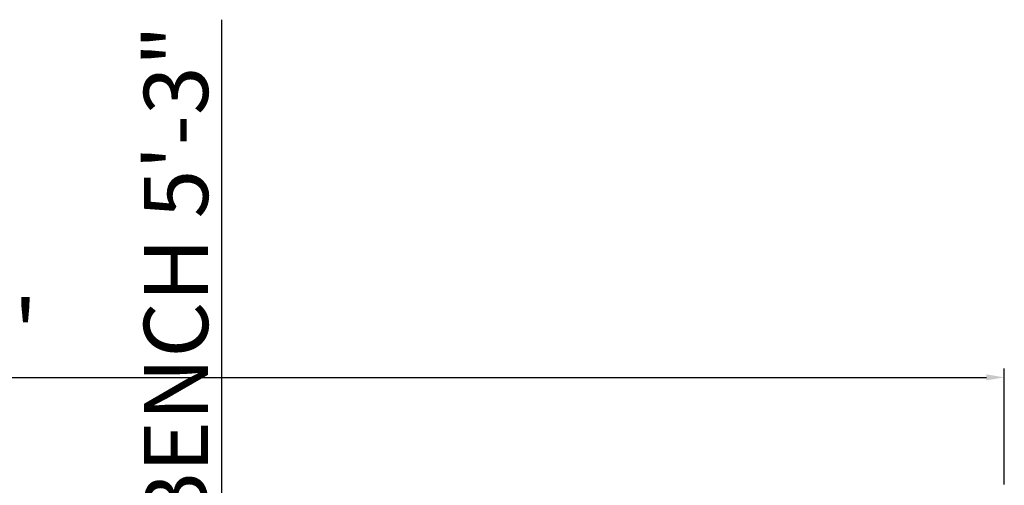
# Model space of a CAD drawing. Units: inches. Extents: x 3148 to 3962, y 1142 to 1671.
# Tile 6 of 9: x 3344 to 3482, y 1555 to 1621. Entities that reach past the tile are written whole.
import ezdxf

# ---------------------------------------------------------------- set-up
doc = ezdxf.new("R2010")
doc.units = ezdxf.units.IN
doc.layers.add('A-ANNO-DIMS', color=2, linetype='Continuous', lineweight=18)
doc.styles.get("Standard").update_dxf_attribs({"font": 'arial.ttf'})
doc.dimstyles.new('ISO-25', dxfattribs={"dimtxt": 9, "dimasz": 2.5, "dimexe": 1.25, "dimexo": 0.625, "dimtad": 1, "dimdec": 1, "dimlunit": 3, "dimtxsty": 'Standard', "dimcen": 2.5, "dimadec": 0, "dimazin": 0, "dimtfac": 1, "dimtdec": 1, "dimtmove": 0, "dimatfit": 3, "dimfxl": 1, "dimarcsym": 0})

# ---------------------------------------------------------------- blocks, each defined once
blk = doc.blocks.new('*D42')
at = {"layer": 'A-ANNO-DIMS', "color": 0, "lineweight": -2, "transparency": 16777216}
for p, q in [((3194.04, 1555.42), (3194.04, 1571.69)), ((3196.54, 1570.44), (3479.54, 1570.44)), ((3482.04, 1555.42), (3482.04, 1571.69))]:
    blk.add_line(p, q, dxfattribs=at)
at = {"layer": 'A-ANNO-DIMS', "color": 0, "transparency": 16777216}
for points in [[(3196.54, 1570.86), (3196.54, 1570.02), (3194.04, 1570.44)], [(3479.54, 1570.86), (3479.54, 1570.02), (3482.04, 1570.44)]]:
    blk.add_solid(points, dxfattribs=at)
at = {"layer": 'Defpoints', "color": 0, "transparency": 16777216}
for p in [(3482.04, 1570.44), (3194.04, 1554.8), (3482.04, 1554.8)]:
    blk.add_point(p, dxfattribs=at)
at = {"layer": 'A-ANNO-DIMS', "color": 0, "transparency": 16777216, "insert": (3338.04, 1575.58), "char_height": 9, "attachment_point": 5}
blk.add_mtext("24'", dxfattribs=at)
blk = doc.blocks.new('*D92')
at = {"layer": 'A-ANNO-DIMS', "color": 0, "lineweight": -2, "transparency": 16777216}
for p, q in [((3372.39, 1545.8), (3372.39, 1620.58)), ((3363.56, 1545.8), (3373.64, 1545.8)), ((3372.39, 1485.31), (3372.39, 1543.3)), ((3363.56, 1482.81), (3373.64, 1482.81))]:
    blk.add_line(p, q, dxfattribs=at)
at = {"layer": 'A-ANNO-DIMS', "color": 0, "transparency": 16777216}
for points in [[(3371.97, 1543.3), (3372.81, 1543.3), (3372.39, 1545.8)], [(3371.97, 1485.31), (3372.81, 1485.31), (3372.39, 1482.81)]]:
    blk.add_solid(points, dxfattribs=at)
at = {"layer": 'Defpoints', "color": 0, "transparency": 16777216}
for p in [(3362.94, 1545.8), (3372.39, 1545.8), (3362.94, 1482.81)]:
    blk.add_point(p, dxfattribs=at)
at = {"layer": 'A-ANNO-DIMS', "color": 0, "transparency": 16777216, "insert": (3367.11, 1584.44), "char_height": 9, "attachment_point": 5, "rotation": 90}
blk.add_mtext('BENCH 5\'-3"', dxfattribs=at)

msp = doc.modelspace()

# ---------------------------------------------------------------- dimensions: what is measured, and where the dimension line sits
at = {"layer": 'A-ANNO-DIMS'}
dim = msp.add_linear_dim(base=(3372.39, 1545.8), p1=(3362.94, 1482.81), p2=(3362.94, 1545.8), angle=90, text='BENCH <>', dimstyle='ISO-25', override={"dimdec": 1, "dimlfac": 1, "dimrnd": 0, "dimzin": 1, "dimdsep": 46, "dimlunit": 4, "dimfrac": 2}, dxfattribs=at)
dim.commit()
dim.dimension.update_dxf_attribs({"geometry": '*D92', "text_midpoint": (3367.11, 1584.44)})
dim = msp.add_linear_dim(base=(3482.04, 1570.44), p1=(3194.04, 1554.8), p2=(3482.04, 1554.8), dimstyle='ISO-25', override={"dimclrd": 0, "dimclre": 0, "dimclrt": 0}, dxfattribs=at)
dim.commit()
dim.dimension.update_dxf_attribs({"geometry": '*D42', "text_midpoint": (3338.04, 1575.58)})

doc.saveas('drawing.dxf')
